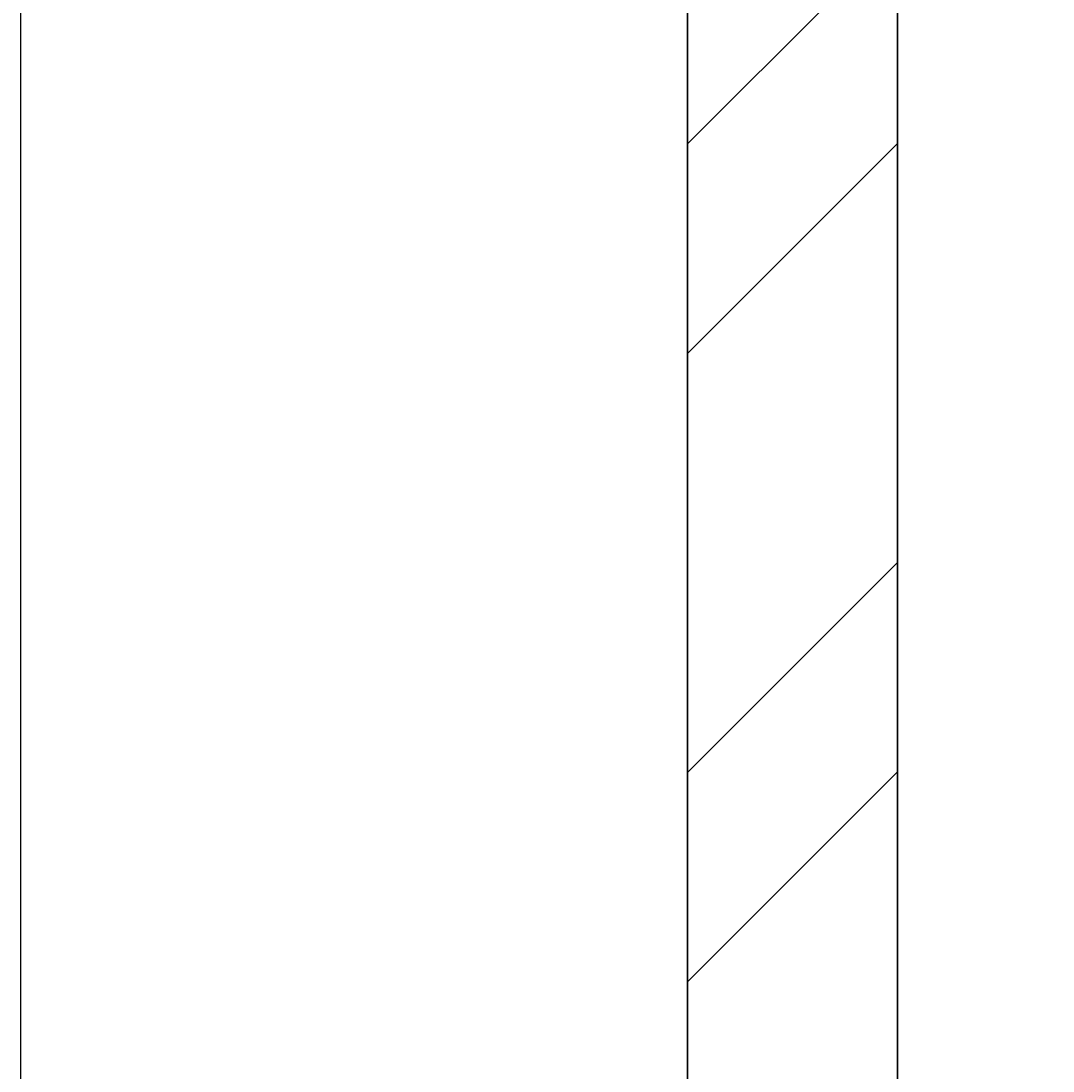
# Model space of a CAD drawing. Units: inches. Extents: x 1962 to 2771, y 1245 to 2660.
# Tile 40 of 114: x 2072.02 to 2094.14, y 2052.97 to 2075.47. Entities that reach past the tile are written whole.
import ezdxf

# ---------------------------------------------------------------- set-up
doc = ezdxf.new("R2010")
doc.units = ezdxf.units.IN
for name, color, linetype, lineweight in [('A-ANNO-DIMS', 2, 'Continuous', 18), ('A-WALL', 7, 'Continuous', 35), ('A-WALL-PATT', 252, 'Continuous', 13)]:
    doc.layers.add(name, color=color, linetype=linetype, lineweight=lineweight)
doc.styles.get("Standard").update_dxf_attribs({"font": 'arial.ttf'})
doc.dimstyles.get("Standard").update_dxf_attribs({"dimtxt": 0.18, "dimasz": 0.18, "dimexe": 0.18, "dimexo": 0.0625, "dimgap": 0.09, "dimtad": 0, "dimtih": 1, "dimtoh": 1, "dimdec": 4, "dimzin": 0, "dimdsep": 46, "dimtxsty": 'Standard', "dimcen": 0.09, "dimadec": 0, "dimazin": 0, "dimtfac": 1, "dimtdec": 4, "dimtofl": 0, "dimtmove": 0, "dimatfit": 3, "dimfxl": 1, "dimtolj": 1, "dimtzin": 0, "dimarcsym": 0})

# ---------------------------------------------------------------- blocks, each defined once
blk = doc.blocks.new('*D40')
at = {"layer": 'A-ANNO-DIMS', "color": 0, "lineweight": -2, "transparency": 16777216}
for p, q in [((2072.02, 2033.906), (2072.02, 2583.474)), ((2660.807, 2524.406), (2660.807, 2583.474)), ((2072.2, 2583.294), (2366.02, 2583.294)), ((2660.627, 2583.294), (2366.808, 2583.294))]:
    blk.add_line(p, q, dxfattribs=at)
at = {"layer": 'A-ANNO-DIMS', "color": 0, "transparency": 16777216}
for points in [[(2072.2, 2583.324), (2072.2, 2583.264), (2072.02, 2583.294)], [(2660.627, 2583.324), (2660.627, 2583.264), (2660.807, 2583.294)]]:
    blk.add_solid(points, dxfattribs=at)
at = {"layer": 'Defpoints', "color": 0, "transparency": 16777216}
for p in [(2660.807, 2583.294), (2660.807, 2524.344), (2072.02, 2033.844)]:
    blk.add_point(p, dxfattribs=at)
at = {"layer": 'A-ANNO-DIMS', "color": 0, "transparency": 16777216, "insert": (2366.414, 2583.294), "char_height": 0.18, "attachment_point": 5}
blk.add_mtext('\\A1;588.8', dxfattribs=at)
blk = doc.blocks.new('*D43')
at = {"layer": 'A-ANNO-DIMS', "color": 0, "lineweight": -2, "transparency": 16777216}
for p, q in [((2086.245, 2524.344), (2012.89, 2524.344)), ((2013.07, 2524.164), (2013.07, 2279.276)), ((2013.07, 2034.024), (2013.07, 2278.912)), ((2071.958, 2033.844), (2012.89, 2033.844))]:
    blk.add_line(p, q, dxfattribs=at)
at = {"layer": 'A-ANNO-DIMS', "color": 0, "transparency": 16777216}
for points in [[(2013.04, 2524.164), (2013.1, 2524.164), (2013.07, 2524.344)], [(2013.04, 2034.024), (2013.1, 2034.024), (2013.07, 2033.844)]]:
    blk.add_solid(points, dxfattribs=at)
at = {"layer": 'Defpoints', "color": 0, "transparency": 16777216}
for p in [(2086.307, 2524.344), (2013.07, 2033.844), (2072.02, 2033.844)]:
    blk.add_point(p, dxfattribs=at)
at = {"layer": 'A-ANNO-DIMS', "color": 0, "transparency": 16777216, "insert": (2013.07, 2279.094), "char_height": 0.18, "attachment_point": 5}
blk.add_mtext('\\A1;490.5', dxfattribs=at)

msp = doc.modelspace()

# ---------------------------------------------------------------- hatches: boundary and pattern name
at = {"layer": 'A-WALL-PATT'}
h = msp.add_hatch(dxfattribs=at)
h.set_pattern_fill('ANSI32', color=256)
h.paths.add_polyline_path([(2090.8074, 2467.3437), (2141.6481, 2467.3437), (2141.6481, 2469.5937), (2141.6481, 2471.8437), (2086.3074, 2471.8437), (2086.3074, 2422.5333), (2090.8074, 2422.5333)])
h.paths.add_polyline_path([(2282.7664, 2471.8437), (2204.8982, 2471.8437), (2204.8982, 2467.3437), (2234.8074, 2467.3437), (2234.8074, 2311.3437), (2228.7492, 2311.3437), (2228.7492, 2306.8437), (2234.8074, 2306.8437), (2331.9227, 2306.8437), (2331.9227, 2309.0937), (2331.9227, 2311.3437), (2239.3074, 2311.3437), (2239.3074, 2467.3437), (2282.7664, 2467.3437), (2282.7664, 2469.5937)])
h.paths.add_polyline_path([(2471.4531, 2519.8437), (2552.011, 2519.8437), (2564.3996, 2519.8437), (2564.3996, 2511.1389), (2568.8996, 2511.1389), (2568.8996, 2524.3437), (2466.9531, 2524.3437), (2466.9531, 2471.8437), (2450.0749, 2471.8437), (2446.4672, 2471.8437), (2446.4672, 2467.3437), (2450.0749, 2467.3437), (2475.9988, 2467.3437), (2475.9988, 2469.5937), (2475.9988, 2471.8437), (2471.4531, 2471.8437)])
h.paths.add_polyline_path([(2575.2231, 2469.5937), (2575.2231, 2471.8437), (2568.8996, 2471.8437), (2568.8996, 2487.1389), (2564.3996, 2487.1389), (2564.3996, 2471.8437), (2556.511, 2471.8437), (2499.2904, 2471.8437), (2499.2904, 2467.3437), (2507.8074, 2467.3437), (2507.8074, 2311.3437), (2414.863, 2311.3437), (2414.863, 2306.8437), (2512.3074, 2306.8437), (2517.0114, 2306.8437), (2517.0114, 2309.0937), (2517.0114, 2311.3437), (2512.3074, 2311.3437), (2512.3074, 2467.3437), (2575.2231, 2467.3437)])
h.paths.add_polyline_path([(2660.8074, 2471.8437), (2600.9602, 2471.8437), (2600.9602, 2467.3437), (2656.3074, 2467.3437), (2656.3074, 2432.5704), (2660.8074, 2432.5704)])
h.paths.add_polyline_path([(2660.8074, 2372.5704), (2656.3074, 2372.5704), (2656.3074, 2311.3437), (2600.276, 2311.3437), (2600.276, 2309.0937), (2600.276, 2306.8437), (2656.3074, 2306.8437), (2656.3074, 2296.2593), (2660.8074, 2296.2593)])
h.paths.add_polyline_path([(2572.3074, 2306.8437), (2577.1385, 2306.8437), (2577.1385, 2311.3437), (2551.082, 2311.3437), (2551.082, 2306.8437), (2567.8074, 2306.8437), (2567.8074, 2258.8437), (2540.0574, 2258.8437), (2540.0574, 2256.5937), (2540.0574, 2254.3437), (2567.8074, 2254.3437), (2656.3074, 2254.3437), (2656.3074, 2236.9085), (2660.8074, 2236.9085), (2660.8074, 2272.2593), (2656.3074, 2272.2593), (2656.3074, 2258.8437), (2572.3074, 2258.8437)])
h.paths.add_polyline_path([(2512.3074, 2254.3437), (2518.8716, 2254.3437), (2518.8716, 2256.5937), (2518.8716, 2258.8437), (2507.8074, 2258.8437), (2507.8074, 2177.8437), (2567.8074, 2177.8437), (2567.8074, 2172.9628), (2572.3074, 2172.9628), (2572.3074, 2177.8437), (2656.3074, 2177.8437), (2656.3074, 2166.4846), (2660.8074, 2166.4846), (2660.8074, 2200.9085), (2656.3074, 2200.9085), (2656.3074, 2182.3437), (2512.3074, 2182.3437)])
h.paths.add_polyline_path([(2656.3074, 2129.8437), (2572.3074, 2129.8437), (2572.3074, 2150.3044), (2570.0574, 2150.3044), (2567.8074, 2150.3044), (2567.8074, 2129.8437), (2507.8074, 2129.8437), (2507.8074, 2116.3027), (2510.0574, 2116.3027), (2512.3074, 2116.3027), (2512.3074, 2125.3437), (2567.8074, 2125.3437), (2572.3074, 2125.3437), (2656.3074, 2125.3437)])
h.paths.add_polyline_path([(2090.8074, 2362.5333), (2086.3074, 2362.5333), (2086.3074, 2298.6242), (2090.8074, 2298.6242), (2090.8074, 2306.8437), (2174.8074, 2306.8437), (2174.8074, 2286.4178), (2179.3074, 2286.4178), (2179.3074, 2306.8437), (2192.8641, 2306.8437), (2192.8641, 2309.0937), (2192.8641, 2311.3437), (2090.8074, 2311.3437)])
h.paths.add_polyline_path([(2209.156, 2258.8437), (2179.3074, 2258.8437), (2179.3074, 2263.2236), (2177.0574, 2263.2236), (2174.8074, 2263.2236), (2174.8074, 2258.8437), (2090.8074, 2258.8437), (2090.8074, 2274.6242), (2086.3074, 2274.6242), (2086.3074, 2238.2967), (2088.5574, 2238.2967), (2090.8074, 2238.2967), (2090.8074, 2254.3437), (2209.156, 2254.3437)])
h.paths.add_polyline_path([(2090.8074, 2177.8437), (2234.8074, 2177.8437), (2234.8074, 2173.1428), (2239.3074, 2173.1428), (2239.3074, 2258.8437), (2230.8442, 2258.8437), (2230.8442, 2256.5937), (2230.8442, 2254.3437), (2234.8074, 2254.3437), (2234.8074, 2182.3437), (2090.8074, 2182.3437), (2090.8074, 2202.2967), (2086.3074, 2202.2967), (2086.3074, 2140.0389), (2090.8074, 2140.0389)])
h.paths.add_polyline_path([(2090.8074, 2080.0389), (2086.3074, 2080.0389), (2086.3074, 2033.8437), (2090.8074, 2033.8437)], flags=17)
h.paths.add_polyline_path([(2244.9405, 2033.8437), (2239.3074, 2033.8437), (2239.3074, 2142.0665), (2237.2592, 2142.0665), (2234.8074, 2142.0665), (2234.8074, 2033.8437), (2090.8074, 2033.8437), (2076.5204, 2033.8437), (2072.0204, 2033.8437), (2072.0204, 2000.4493), (2076.5204, 2000.4493), (2076.5204, 2029.3437), (2090.8074, 2029.3437), (2244.9405, 2029.3437), (2244.9405, 2031.5937)])
h.paths.add_polyline_path([(2234.8074, 1933.3437), (2076.5204, 1933.3437), (2076.5204, 1952.4493), (2074.2704, 1952.4493), (2072.0204, 1952.4493), (2072.0204, 1933.3437), (2072.0204, 1928.8437), (2234.8074, 1928.8437)])
h.paths.add_polyline_path([(2090.8074, 1928.8437), (2086.3074, 1928.8437), (2086.3074, 1906.5013), (2090.8074, 1906.5013)])
h.paths.add_polyline_path([(2090.8074, 1846.5013), (2086.3074, 1846.5013), (2086.3074, 1769.9917), (2088.5574, 1769.9917), (2090.8074, 1769.9917), (2090.8074, 1780.3437), (2234.8074, 1780.3437), (2234.8074, 1708.3437), (2230.3764, 1708.3437), (2230.3764, 1703.8437), (2239.3074, 1703.8437), (2239.3074, 1792.6669), (2237.0574, 1792.6669), (2234.8074, 1792.6669), (2234.8074, 1784.8437), (2090.8074, 1784.8437)])
h.paths.add_polyline_path([(2239.3074, 1928.8437), (2244.9405, 1928.8437), (2244.9405, 1931.0937), (2244.9405, 1933.3437), (2234.8074, 1933.3437), (2234.8074, 1928.8437), (2234.8074, 1825.5949), (2239.3074, 1825.5949)])
h.paths.add_polyline_path([(2148.0425, 1649.0937), (2148.0425, 1651.3437), (2090.8074, 1651.3437), (2090.8074, 1646.8437), (2148.0425, 1646.8437)], flags=0)
h.paths.add_polyline_path([(2207.5601, 1708.3437), (2090.8074, 1708.3437), (2090.8074, 1703.8437), (2174.8074, 1703.8437), (2174.8074, 1651.3437), (2170.4457, 1651.3437), (2170.4457, 1646.8437), (2195.9924, 1646.8437), (2195.9924, 1649.0937), (2195.9924, 1651.3437), (2179.3074, 1651.3437), (2179.3074, 1703.8437), (2207.5601, 1703.8437), (2207.5601, 1706.0937)])
h.paths.add_polyline_path([(2090.8074, 1733.9917), (2086.3074, 1733.9917), (2086.3074, 1696.1032), (2088.5574, 1696.1032), (2090.8074, 1696.1032)])
h.paths.add_polyline_path([(2090.8074, 1672.1032), (2086.3074, 1672.1032), (2086.3074, 1600.3335), (2090.8074, 1600.3335)])
h.paths.add_polyline_path([(2090.8074, 1540.3335), (2086.3074, 1540.3335), (2086.3074, 1486.3437), (2139.6766, 1486.3437), (2139.6766, 1490.8437), (2090.8074, 1490.8437)])
h.paths.add_polyline_path([(2302.3876, 1490.8437), (2239.3074, 1490.8437), (2239.3074, 1646.8437), (2335.9994, 1646.8437), (2335.9994, 1651.3437), (2229.884, 1651.3437), (2229.884, 1646.8437), (2234.8074, 1646.8437), (2234.8074, 1490.8437), (2202.7103, 1490.8437), (2202.7103, 1488.5937), (2202.7103, 1486.3437), (2275.0699, 1486.3437), (2275.0699, 1475.772), (2279.5699, 1475.772), (2279.5699, 1486.3437), (2302.3876, 1486.3437)])
h.paths.add_polyline_path([(2279.5699, 1451.772), (2275.0699, 1451.772), (2275.0699, 1438.3437), (2174.8074, 1438.3437), (2174.8074, 1486.3437), (2179.7922, 1486.3437), (2179.7922, 1490.8437), (2163.3585, 1490.8437), (2163.3585, 1488.5937), (2163.3585, 1486.3437), (2170.3074, 1486.3437), (2170.3074, 1433.8437), (2279.5699, 1433.8437)])
h.paths.add_polyline_path([(2427.2363, 1490.8437), (2375.8074, 1490.8437), (2375.8074, 1646.8437), (2381.6401, 1646.8437), (2381.6401, 1651.3437), (2365.887, 1651.3437), (2365.887, 1649.0937), (2365.887, 1646.8437), (2371.3074, 1646.8437), (2371.3074, 1490.8437), (2327.5627, 1490.8437), (2327.5627, 1488.5937), (2327.5627, 1486.3437), (2371.3074, 1486.3437), (2371.3074, 1433.8437), (2375.8074, 1433.8437), (2375.8074, 1486.3437), (2427.2363, 1486.3437)])
h.paths.add_polyline_path([(2512.3074, 1646.8437), (2519.4351, 1646.8437), (2519.4351, 1649.0937), (2519.4351, 1651.3437), (2507.8074, 1651.3437), (2416.0063, 1651.3437), (2416.0063, 1649.0937), (2416.0063, 1646.8437), (2507.8074, 1646.8437), (2507.8074, 1490.8437), (2497.0532, 1490.8437), (2497.0532, 1488.5937), (2497.0532, 1486.3437), (2574.9344, 1486.3437), (2574.9344, 1476.0181), (2579.4344, 1476.0181), (2579.4344, 1486.3437), (2584.4872, 1486.3437), (2584.3074, 1490.8437), (2512.3074, 1490.8437)])
h.paths.add_polyline_path([(2470.5091, 1486.3437), (2473.9767, 1486.3437), (2473.9767, 1490.8437), (2449.6605, 1490.8437), (2449.6605, 1488.5937), (2449.6605, 1486.3437), (2466.0091, 1486.3437), (2466.0091, 1433.8437), (2470.5091, 1433.8437), (2579.4344, 1433.8437), (2579.4344, 1452.0181), (2574.9344, 1452.0181), (2574.9344, 1438.3437), (2554.5091, 1438.3437), (2470.5091, 1438.3437)])
h.paths.add_polyline_path([(2656.3074, 1490.8437), (2611.86, 1490.8437), (2611.86, 1486.3437), (2656.3074, 1486.3437)])
h.paths.add_polyline_path([(2660.8074, 1532.7007), (2658.5574, 1532.7007), (2656.3074, 1532.7007), (2656.3074, 1486.3437), (2660.8074, 1486.3437)])
h.paths.add_polyline_path([(2660.8074, 1664.9663), (2656.3074, 1664.9663), (2656.3074, 1651.3437), (2602.2313, 1651.3437), (2602.2313, 1646.8437), (2656.3074, 1646.8437), (2656.3074, 1592.7007), (2660.8074, 1592.7007)])
h.paths.add_polyline_path([(2660.8074, 1724.5221), (2656.3074, 1724.5221), (2656.3074, 1703.8437), (2542.4725, 1703.8437), (2542.4725, 1699.3437), (2567.8074, 1699.3437), (2567.8074, 1651.3437), (2552.7766, 1651.3437), (2552.7766, 1649.0937), (2552.7766, 1646.8437), (2577.2878, 1646.8437), (2577.2878, 1649.0937), (2577.2878, 1651.3437), (2572.3074, 1651.3437), (2572.3074, 1699.3437), (2656.3074, 1699.3437), (2656.3074, 1688.9663), (2660.8074, 1688.9663)])
h.paths.add_polyline_path([(2660.8074, 1880.6524), (2656.3074, 1880.6524), (2656.3074, 1832.8437), (2512.3074, 1832.8437), (2512.3074, 1837.8959), (2507.8074, 1837.8959), (2507.8074, 1828.3437), (2567.8074, 1828.3437), (2567.8074, 1804.3437), (2572.3074, 1804.3437), (2572.3074, 1828.3437), (2656.3074, 1828.3437), (2656.3074, 1818.6778), (2660.8074, 1818.6778)])
h.paths.add_polyline_path([(2660.8074, 1794.6778), (2656.3074, 1794.6778), (2656.3074, 1780.3437), (2572.3074, 1780.3437), (2572.3074, 1783.0303), (2570.0574, 1783.0303), (2567.8074, 1783.0303), (2567.8074, 1780.3437), (2507.8074, 1780.3437), (2507.8074, 1699.3437), (2517.8858, 1699.3437), (2517.8858, 1701.5937), (2517.8858, 1703.8437), (2512.3074, 1703.8437), (2512.3074, 1775.8437), (2656.3074, 1775.8437), (2656.3074, 1760.5221), (2660.8074, 1760.5221)])
h.paths.add_polyline_path([(2660.8074, 1981.3437), (2660.8074, 2020.2808), (2658.5574, 2020.2808), (2656.3074, 2020.2808), (2656.3074, 1981.3437), (2512.3074, 1981.3437), (2512.3074, 2086.6996), (2507.8074, 2086.6996), (2507.8074, 1981.3437), (2375.8074, 1981.3437), (2375.8074, 1986.8505), (2373.5574, 1986.8505), (2371.3074, 1986.8505), (2371.3074, 1973.2607), (2375.8074, 1973.2607), (2375.8074, 1976.8437), (2507.8074, 1976.8437), (2507.8074, 1865.4281), (2510.0574, 1865.4281), (2512.3074, 1865.4281), (2512.3074, 1976.8437), (2660.8074, 1976.8437)])
h.paths.add_polyline_path([(2375.8074, 1940.297), (2373.5574, 1940.297), (2371.3074, 1940.297), (2371.3074, 1933.3437), (2278.4434, 1933.3437), (2278.4434, 1928.8437), (2371.3074, 1928.8437), (2371.3074, 1651.3437), (2375.8074, 1651.3437)])
h.paths.add_polyline_path([(2660.8074, 1976.8437), (2656.3074, 1976.8437), (2656.3074, 1940.6524), (2660.8074, 1940.6524)], flags=17)
h.paths.add_polyline_path([(2660.8074, 2142.4846), (2656.3074, 2142.4846), (2656.3074, 2080.2808), (2660.8074, 2080.2808)])
h.paths.add_polyline_path([(2381.4189, 2311.3437), (2375.8074, 2311.3437), (2375.8074, 2467.3437), (2424.7242, 2467.3437), (2424.7242, 2469.5937), (2424.7242, 2471.8437), (2375.8074, 2471.8437), (2375.8074, 2524.3437), (2371.3074, 2524.3437), (2371.3074, 2471.8437), (2307.2097, 2471.8437), (2307.2097, 2467.3437), (2371.3074, 2467.3437), (2371.3074, 2311.3437), (2366.8901, 2311.3437), (2366.8901, 2306.8437), (2371.3074, 2306.8437), (2371.3074, 2033.8437), (2279.6589, 2033.8437), (2279.6589, 2029.3437), (2371.3074, 2029.3437), (2371.3074, 2014.2598), (2375.8074, 2014.2598), (2375.8074, 2306.8437), (2381.4189, 2306.8437)])
h.paths.add_polyline_path([(2263.3074, 2524.3437), (2170.3074, 2524.3437), (2170.3074, 2519.8437), (2170.3074, 2471.8437), (2165.0312, 2471.8437), (2165.0312, 2467.3437), (2179.6721, 2467.3437), (2179.6721, 2469.5161), (2179.6721, 2471.8437), (2174.8074, 2471.8437), (2174.8074, 2519.8437), (2258.8074, 2519.8437), (2258.8074, 2511.6436), (2263.3074, 2511.6436)])
h.paths.add_polyline_path([(2245.0232, 1361.4123), (2492.9468, 1361.4123), (2492.9468, 1398.505), (2245.0232, 1398.505)], flags=9)
h.paths.add_polyline_path([(2388.1434, 2086.6936), (2425.0704, 2086.6936), (2425.0704, 2105.3509), (2388.1434, 2105.3509)], flags=9)
h.paths.add_polyline_path([(2404.922, 2242.6744), (2445.7337, 2242.6744), (2445.7337, 2261.3318), (2404.922, 2261.3318)], flags=9)
h.paths.add_polyline_path([(2269.4107, 2156.7935), (2306.3378, 2156.7935), (2306.3378, 2175.4508), (2269.4107, 2175.4508)], flags=9)
h.paths.add_polyline_path([(2269.3277, 2233.4343), (2306.2547, 2233.4343), (2306.2547, 2252.0917), (2269.3277, 2252.0917)], flags=9)
h.paths.add_polyline_path([(2431.6052, 2320.6922), (2470.4456, 2320.6922), (2470.4456, 2339.3495), (2431.6052, 2339.3495)], flags=25)
h.paths.add_polyline_path([(2249.6902, 2315.7608), (2288.5306, 2315.7608), (2288.5306, 2334.4182), (2249.6902, 2334.4182)], flags=25)
h.paths.add_polyline_path([(2096.9301, 2314.3181), (2135.7704, 2314.3181), (2135.7704, 2332.9755), (2096.9301, 2332.9755)], flags=25)
h.paths.add_polyline_path([(2134.3475, 2285.7089), (2161.4655, 2285.7089), (2161.4655, 2304.3662), (2134.3475, 2304.3662)], flags=9)
h.paths.add_polyline_path([(2126.5155, 2209.4076), (2159.9227, 2209.4076), (2159.9227, 2228.065), (2126.5155, 2228.065)], flags=25)
h.paths.add_polyline_path([(2110.5753, 2141.5299), (2149.4157, 2141.5299), (2149.4157, 2160.1872), (2110.5753, 2160.1872)], flags=25)
h.paths.add_polyline_path([(2249.8618, 1968.3317), (2286.3966, 1968.3317), (2286.3966, 1986.989), (2249.8618, 1986.989)], flags=9)
h.paths.add_polyline_path([(2395.9507, 1777.0051), (2436.7624, 1777.0051), (2436.7624, 1795.6625), (2395.9507, 1795.6625)], flags=9)
h.paths.add_polyline_path([(2398.5259, 1888.5651), (2435.0062, 1888.5651), (2435.0062, 1907.2224), (2398.5259, 1907.2224)], flags=25)
h.paths.add_polyline_path([(2259.3506, 1728.3559), (2296.2776, 1728.3559), (2296.2776, 1747.0132), (2259.3506, 1747.0132)], flags=9)
h.paths.add_polyline_path([(2271.3698, 1845.268), (2308.2968, 1845.268), (2308.2968, 1863.9253), (2271.3698, 1863.9253)], flags=9)
h.paths.add_polyline_path([(2120.9355, 1786.3027), (2159.7759, 1786.3027), (2159.7759, 1804.9601), (2120.9355, 1804.9601)], flags=25)
h.paths.add_polyline_path([(2121.3164, 1732.1043), (2154.7236, 1732.1043), (2154.7236, 1750.7616), (2121.3164, 1750.7616)], flags=25)
h.paths.add_polyline_path([(2118.3706, 1678.8997), (2147.5282, 1678.8997), (2147.5282, 1697.557), (2118.3706, 1697.557)], flags=25)
h.paths.add_polyline_path([(2385.9227, 1493.557), (2424.763, 1493.557), (2424.763, 1512.2143), (2385.9227, 1512.2143)], flags=25)
h.paths.add_polyline_path([(2248.7058, 1500.0256), (2287.5462, 1500.0256), (2287.5462, 1518.6829), (2248.7058, 1518.6829)], flags=25)
h.paths.add_polyline_path([(2104.1669, 1617.3771), (2143.0073, 1617.3771), (2143.0073, 1636.0344), (2104.1669, 1636.0344)], flags=9)
h.paths.add_polyline_path([(2096.0714, 1447.8824), (2137.3845, 1447.8824), (2137.3845, 1458.1859), (2096.0714, 1458.1859)], flags=9)
h.paths.add_polyline_path([(2180.6114, 1440.325), (2209.7689, 1440.325), (2209.7689, 1458.9823), (2180.6114, 1458.9823)], flags=25)
h.paths.add_polyline_path([(2316.1698, 1447.9637), (2357.4829, 1447.9637), (2357.4829, 1458.2673), (2316.1698, 1458.2673)], flags=9)
h.paths.add_polyline_path([(2397.6187, 1447.9637), (2438.9318, 1447.9637), (2438.9318, 1458.2673), (2397.6187, 1458.2673)], flags=9)
h.paths.add_polyline_path([(2473.0778, 1439.5953), (2502.2354, 1439.5953), (2502.2354, 1458.2527), (2473.0778, 1458.2527)], flags=25)
h.paths.add_polyline_path([(2589.7027, 1447.8819), (2631.0158, 1447.8819), (2631.0158, 1458.1855), (2589.7027, 1458.1855)], flags=9)
h.paths.add_polyline_path([(2522.4009, 1497.5285), (2561.2413, 1497.5285), (2561.2413, 1516.1859), (2522.4009, 1516.1859)], flags=25)
h.paths.add_polyline_path([(2579.6565, 1671.3482), (2608.8141, 1671.3482), (2608.8141, 1690.0056), (2579.6565, 1690.0056)], flags=25)
h.paths.add_polyline_path([(2544.7038, 1725.5064), (2578.1111, 1725.5064), (2578.1111, 1744.1637), (2544.7038, 1744.1637)], flags=25)
h.paths.add_polyline_path([(2578.1191, 1807.472), (2607.2766, 1807.472), (2607.2766, 1826.1293), (2578.1191, 1826.1293)], flags=25)
h.paths.add_polyline_path([(2595.0614, 1835.1839), (2633.9018, 1835.1839), (2633.9018, 1853.8413), (2595.0614, 1853.8413)], flags=25)
h.paths.add_polyline_path([(2567.0097, 2097.7035), (2605.8501, 2097.7035), (2605.8501, 2116.3609), (2567.0097, 2116.3609)], flags=9)
h.paths.add_polyline_path([(2586.644, 2134.6454), (2615.8015, 2134.6454), (2615.8015, 2153.3027), (2586.644, 2153.3027)], flags=9)
h.paths.add_polyline_path([(2544.6185, 2212.6783), (2578.0258, 2212.6783), (2578.0258, 2231.3356), (2544.6185, 2231.3356)], flags=25)
h.paths.add_polyline_path([(2577.0273, 2256.9023), (2606.1849, 2256.9023), (2606.1849, 2275.5597), (2577.0273, 2275.5597)], flags=24)
h.paths.add_polyline_path([(2605.2683, 2315.2821), (2644.1087, 2315.2821), (2644.1087, 2333.9395), (2605.2683, 2333.9395)], flags=25)
h.paths.add_polyline_path([(2583.1244, 2496.1815), (2624.4375, 2496.1815), (2624.4375, 2506.4851), (2583.1244, 2506.4851)], flags=9)
h.paths.add_polyline_path([(2474.761, 2497.0823), (2503.9185, 2497.0823), (2503.9185, 2515.7397), (2474.761, 2515.7397)], flags=25)
h.paths.add_polyline_path([(2387.5787, 2494.2563), (2428.902, 2494.2563), (2428.902, 2504.5598), (2387.5787, 2504.5598)], flags=9)
h.paths.add_polyline_path([(2300.1657, 2500.1564), (2341.4788, 2500.1564), (2341.4788, 2510.46), (2300.1657, 2510.46)], flags=25)
h.paths.add_polyline_path([(2176.8589, 2497.5843), (2206.0165, 2497.5843), (2206.0165, 2516.2416), (2176.8589, 2516.2416)], flags=25)
h.paths.add_polyline_path([(2097.4668, 2494.9762), (2138.7799, 2494.9762), (2138.7799, 2505.2798), (2097.4668, 2505.2798)], flags=9)

# ---------------------------------------------------------------- linework, layer by layer
at = {"layer": 'A-WALL'}
for p, q in [((2086.3074, 2471.8437), (2086.3074, 2033.8437)), ((2090.8074, 2177.8437), (2090.8074, 2033.8437))]:
    msp.add_line(p, q, dxfattribs=at)

# ---------------------------------------------------------------- dimensions: what is measured, and where the dimension line sits
at = {"layer": 'A-ANNO-DIMS'}
dim = msp.add_linear_dim(base=(2660.8074, 2583.2937), p1=(2072.0204, 2033.8437), p2=(2660.8074, 2524.3437), dimstyle='Standard', override={"dimdec": 1, "dimlfac": 1, "dimrnd": 0, "dimzin": 0, "dimdsep": 46, "dimlunit": 2}, dxfattribs=at)
dim.commit()
dim.dimension.update_dxf_attribs({"geometry": '*D40', "text_midpoint": (2366.4139, 2583.2937)})
dim = msp.add_linear_dim(base=(2013.0704, 2033.8437), p1=(2086.3074, 2524.3437), p2=(2072.0204, 2033.8437), angle=90, dimstyle='Standard', override={"dimdec": 1, "dimlfac": 1, "dimrnd": 0, "dimzin": 0, "dimdsep": 46, "dimlunit": 2}, dxfattribs=at)
dim.commit()
dim.dimension.update_dxf_attribs({"geometry": '*D43', "text_midpoint": (2013.0704, 2279.0937)})

doc.saveas('drawing.dxf')
